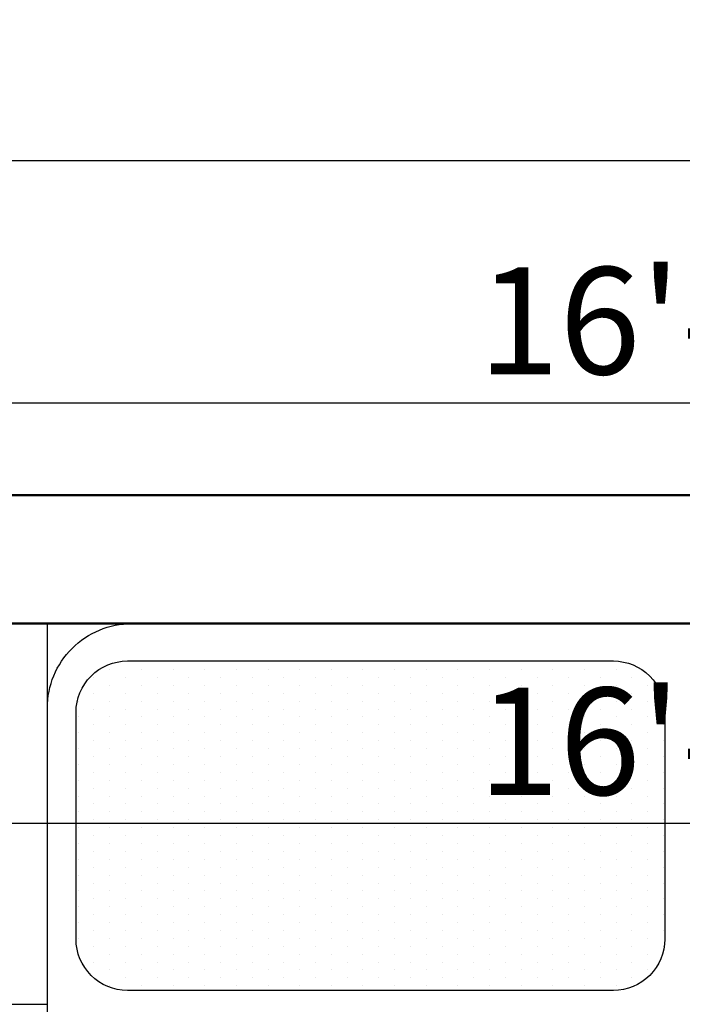
# Model space of a CAD drawing. Units: inches. Extents: x 3064 to 19385, y 846 to 15425.
# Tile 105 of 108: x 7734 to 7765, y 1373 to 1419. Entities that reach past the tile are written whole.
import ezdxf

# ---------------------------------------------------------------- set-up
doc = ezdxf.new("R2010")
doc.units = ezdxf.units.IN
for name, color, linetype, lineweight in [('A-ANNO-DIMS', 2, 'Continuous', 18), ('A-FLOR-FIXT', 9, 'Continuous', 18), ('A-WALL', 7, 'Continuous', 50)]:
    doc.layers.add(name, color=color, linetype=linetype, lineweight=lineweight)
doc.layers.add('BLOCK', color=6, linetype='Continuous')
doc.styles.get("Standard").update_dxf_attribs({"font": 'arial.ttf'})
doc.dimstyles.new('ISO-25', dxfattribs={"dimtxt": 9, "dimasz": 2.5, "dimexe": 1.25, "dimexo": 0.625, "dimtad": 1, "dimdec": 1, "dimlunit": 3, "dimtxsty": 'Standard', "dimcen": 2.5, "dimadec": 0, "dimazin": 0, "dimtfac": 1, "dimtdec": 1, "dimtmove": 0, "dimatfit": 3, "dimfxl": 1, "dimarcsym": 0})

# ---------------------------------------------------------------- blocks, each defined once
blk = doc.blocks.new('*D338')
at = {"layer": 'A-ANNO-DIMS', "color": 0, "lineweight": -2, "transparency": 16777216}
for p, q in [((7667.246, 1396.965), (7667.246, 1401.902)), ((7862.246, 1396.965), (7862.246, 1401.902)), ((7669.746, 1400.652), (7859.746, 1400.652))]:
    blk.add_line(p, q, dxfattribs=at)
at = {"layer": 'A-ANNO-DIMS', "color": 0, "transparency": 16777216}
for points in [[(7669.746, 1401.069), (7669.746, 1400.235), (7667.246, 1400.652)], [(7859.746, 1401.069), (7859.746, 1400.235), (7862.246, 1400.652)]]:
    blk.add_solid(points, dxfattribs=at)
at = {"layer": 'Defpoints', "color": 0, "transparency": 16777216}
for p in [(7862.246, 1400.652), (7667.246, 1396.34), (7862.246, 1396.34)]:
    blk.add_point(p, dxfattribs=at)
at = {"layer": 'A-ANNO-DIMS', "color": 0, "transparency": 16777216, "insert": (7764.746, 1403.832), "char_height": 5, "attachment_point": 5}
blk.add_mtext('16\'-3"', dxfattribs=at)
blk = doc.blocks.new('*D226')
at = {"layer": 'A-ANNO-DIMS', "color": 0, "lineweight": -2, "transparency": 16777216}
for p, q in [((7526.246, 1396.965), (7526.246, 1413.199)), ((7868.246, 1396.965), (7868.246, 1413.199)), ((7865.746, 1411.949), (7528.746, 1411.949))]:
    blk.add_line(p, q, dxfattribs=at)
at = {"layer": 'A-ANNO-DIMS', "color": 0, "transparency": 16777216}
for points in [[(7528.746, 1412.366), (7528.746, 1411.533), (7526.246, 1411.949)], [(7865.746, 1412.366), (7865.746, 1411.533), (7868.246, 1411.949)]]:
    blk.add_solid(points, dxfattribs=at)
at = {"layer": 'Defpoints', "color": 0, "transparency": 16777216}
for p in [(7526.246, 1411.949), (7526.246, 1396.34), (7868.246, 1396.34)]:
    blk.add_point(p, dxfattribs=at)
at = {"layer": 'A-ANNO-DIMS', "color": 0, "transparency": 16777216, "insert": (7697.246, 1415.127), "char_height": 5, "attachment_point": 5}
blk.add_mtext('28\'-6"', dxfattribs=at)
blk = doc.blocks.new('*D248')
at = {"layer": 'A-ANNO-DIMS', "color": 0, "lineweight": -2, "transparency": 16777216}
for p, q in [((7667.246, 1389.715), (7667.246, 1379.771)), ((7862.246, 1389.715), (7862.246, 1379.771)), ((7669.746, 1381.021), (7859.746, 1381.021))]:
    blk.add_line(p, q, dxfattribs=at)
at = {"layer": 'A-ANNO-DIMS', "color": 0, "transparency": 16777216}
for points in [[(7669.746, 1381.437), (7669.746, 1380.604), (7667.246, 1381.021)], [(7859.746, 1381.437), (7859.746, 1380.604), (7862.246, 1381.021)]]:
    blk.add_solid(points, dxfattribs=at)
at = {"layer": 'Defpoints', "color": 0, "transparency": 16777216}
for p in [(7667.246, 1390.34), (7862.246, 1390.34), (7862.246, 1381.021)]:
    blk.add_point(p, dxfattribs=at)
at = {"layer": 'A-ANNO-DIMS', "color": 0, "transparency": 16777216, "insert": (7764.746, 1384.2), "char_height": 5, "attachment_point": 5}
blk.add_mtext('16\'-3"', dxfattribs=at)
blk = doc.blocks.new('*X7')
at = {"color": 0}
for p, q in [((266.4375, 457.03125), (266.4375, 457.03125)), ((266.8125, 457.03125), (266.8125, 457.03125)), ((267.1875, 457.03125), (267.1875, 457.03125)), ((267.5625, 457.03125), (267.5625, 457.03125)), ((267.9375, 457.03125), (267.9375, 457.03125)), ((268.3125, 457.03125), (268.3125, 457.03125)), ((268.6875, 457.03125), (268.6875, 457.03125)), ((269.0625, 457.03125), (269.0625, 457.03125)), ((269.4375, 457.03125), (269.4375, 457.03125)), ((269.8125, 457.03125), (269.8125, 457.03125)), ((270.1875, 457.03125), (270.1875, 457.03125)), ((270.5625, 457.03125), (270.5625, 457.03125)), ((270.9375, 457.03125), (270.9375, 457.03125)), ((271.3125, 457.03125), (271.3125, 457.03125)), ((271.6875, 457.03125), (271.6875, 457.03125)), ((272.0625, 457.03125), (272.0625, 457.03125)), ((266.25, 456.9375), (266.25, 456.9375)), ((266.625, 456.9375), (266.625, 456.9375)), ((267, 456.9375), (267, 456.9375)), ((267.375, 456.9375), (267.375, 456.9375)), ((267.75, 456.9375), (267.75, 456.9375)), ((268.125, 456.9375), (268.125, 456.9375)), ((268.5, 456.9375), (268.5, 456.9375)), ((268.875, 456.9375), (268.875, 456.9375)), ((269.25, 456.9375), (269.25, 456.9375)), ((269.625, 456.9375), (269.625, 456.9375)), ((270, 456.9375), (270, 456.9375)), ((270.375, 456.9375), (270.375, 456.9375)), ((270.75, 456.9375), (270.75, 456.9375)), ((271.125, 456.9375), (271.125, 456.9375)), ((271.5, 456.9375), (271.5, 456.9375)), ((271.875, 456.9375), (271.875, 456.9375)), ((272.25, 456.9375), (272.25, 456.9375)), ((266.0625, 456.84375), (266.0625, 456.84375)), ((266.25, 456.75), (266.25, 456.75)), ((266.4375, 456.84375), (266.4375, 456.84375)), ((266.625, 456.75), (266.625, 456.75)), ((266.8125, 456.84375), (266.8125, 456.84375)), ((267, 456.75), (267, 456.75)), ((267.1875, 456.84375), (267.1875, 456.84375)), ((267.375, 456.75), (267.375, 456.75)), ((267.5625, 456.84375), (267.5625, 456.84375)), ((267.75, 456.75), (267.75, 456.75)), ((267.9375, 456.84375), (267.9375, 456.84375)), ((268.125, 456.75), (268.125, 456.75)), ((268.3125, 456.84375), (268.3125, 456.84375)), ((268.5, 456.75), (268.5, 456.75)), ((268.6875, 456.84375), (268.6875, 456.84375)), ((268.875, 456.75), (268.875, 456.75)), ((269.0625, 456.84375), (269.0625, 456.84375)), ((269.25, 456.75), (269.25, 456.75)), ((269.4375, 456.84375), (269.4375, 456.84375)), ((269.625, 456.75), (269.625, 456.75)), ((269.8125, 456.84375), (269.8125, 456.84375)), ((270, 456.75), (270, 456.75)), ((270.1875, 456.84375), (270.1875, 456.84375)), ((270.375, 456.75), (270.375, 456.75)), ((270.5625, 456.84375), (270.5625, 456.84375)), ((270.75, 456.75), (270.75, 456.75)), ((270.9375, 456.84375), (270.9375, 456.84375)), ((271.125, 456.75), (271.125, 456.75)), ((271.3125, 456.84375), (271.3125, 456.84375)), ((271.5, 456.75), (271.5, 456.75)), ((271.6875, 456.84375), (271.6875, 456.84375)), ((271.875, 456.75), (271.875, 456.75)), ((272.0625, 456.84375), (272.0625, 456.84375)), ((272.25, 456.75), (272.25, 456.75)), ((272.4375, 456.84375), (272.4375, 456.84375)), ((272.625, 456.75), (272.625, 456.75)), ((266.0625, 456.65625), (266.0625, 456.65625)), ((266.4375, 456.65625), (266.4375, 456.65625)), ((266.8125, 456.65625), (266.8125, 456.65625)), ((267.1875, 456.65625), (267.1875, 456.65625)), ((267.5625, 456.65625), (267.5625, 456.65625)), ((267.9375, 456.65625), (267.9375, 456.65625)), ((268.3125, 456.65625), (268.3125, 456.65625)), ((268.6875, 456.65625), (268.6875, 456.65625)), ((269.0625, 456.65625), (269.0625, 456.65625)), ((269.4375, 456.65625), (269.4375, 456.65625)), ((269.8125, 456.65625), (269.8125, 456.65625)), ((270.1875, 456.65625), (270.1875, 456.65625)), ((270.5625, 456.65625), (270.5625, 456.65625)), ((270.9375, 456.65625), (270.9375, 456.65625)), ((271.3125, 456.65625), (271.3125, 456.65625)), ((271.6875, 456.65625), (271.6875, 456.65625)), ((272.0625, 456.65625), (272.0625, 456.65625)), ((272.4375, 456.65625), (272.4375, 456.65625)), ((265.875, 456.5625), (265.875, 456.5625)), ((266.25, 456.5625), (266.25, 456.5625)), ((266.625, 456.5625), (266.625, 456.5625)), ((267, 456.5625), (267, 456.5625)), ((267.375, 456.5625), (267.375, 456.5625)), ((267.75, 456.5625), (267.75, 456.5625)), ((268.125, 456.5625), (268.125, 456.5625)), ((268.5, 456.5625), (268.5, 456.5625)), ((268.875, 456.5625), (268.875, 456.5625)), ((269.25, 456.5625), (269.25, 456.5625)), ((269.625, 456.5625), (269.625, 456.5625)), ((270, 456.5625), (270, 456.5625)), ((270.375, 456.5625), (270.375, 456.5625)), ((270.75, 456.5625), (270.75, 456.5625)), ((271.125, 456.5625), (271.125, 456.5625)), ((271.5, 456.5625), (271.5, 456.5625)), ((271.875, 456.5625), (271.875, 456.5625)), ((272.25, 456.5625), (272.25, 456.5625)), ((272.625, 456.5625), (272.625, 456.5625)), ((266.0625, 456.46875), (266.0625, 456.46875)), ((266.4375, 456.46875), (266.4375, 456.46875)), ((266.8125, 456.46875), (266.8125, 456.46875)), ((267.1875, 456.46875), (267.1875, 456.46875)), ((267.5625, 456.46875), (267.5625, 456.46875)), ((267.9375, 456.46875), (267.9375, 456.46875)), ((268.3125, 456.46875), (268.3125, 456.46875)), ((268.6875, 456.46875), (268.6875, 456.46875)), ((269.0625, 456.46875), (269.0625, 456.46875)), ((269.4375, 456.46875), (269.4375, 456.46875)), ((269.8125, 456.46875), (269.8125, 456.46875)), ((270.1875, 456.46875), (270.1875, 456.46875)), ((270.5625, 456.46875), (270.5625, 456.46875)), ((270.9375, 456.46875), (270.9375, 456.46875)), ((271.3125, 456.46875), (271.3125, 456.46875)), ((271.6875, 456.46875), (271.6875, 456.46875)), ((272.0625, 456.46875), (272.0625, 456.46875)), ((272.4375, 456.46875), (272.4375, 456.46875)), ((272.8125, 456.46875), (272.8125, 456.46875)), ((265.875, 456.375), (265.875, 456.375)), ((266.0625, 456.28125), (266.0625, 456.28125)), ((266.25, 456.375), (266.25, 456.375)), ((266.4375, 456.28125), (266.4375, 456.28125)), ((266.625, 456.375), (266.625, 456.375)), ((266.8125, 456.28125), (266.8125, 456.28125)), ((267, 456.375), (267, 456.375)), ((267.1875, 456.28125), (267.1875, 456.28125)), ((267.375, 456.375), (267.375, 456.375)), ((267.5625, 456.28125), (267.5625, 456.28125)), ((267.75, 456.375), (267.75, 456.375)), ((267.9375, 456.28125), (267.9375, 456.28125)), ((268.125, 456.375), (268.125, 456.375)), ((268.3125, 456.28125), (268.3125, 456.28125)), ((268.5, 456.375), (268.5, 456.375)), ((268.6875, 456.28125), (268.6875, 456.28125)), ((268.875, 456.375), (268.875, 456.375)), ((269.0625, 456.28125), (269.0625, 456.28125)), ((269.25, 456.375), (269.25, 456.375)), ((269.4375, 456.28125), (269.4375, 456.28125)), ((269.625, 456.375), (269.625, 456.375)), ((269.8125, 456.28125), (269.8125, 456.28125)), ((270, 456.375), (270, 456.375)), ((270.1875, 456.28125), (270.1875, 456.28125)), ((270.375, 456.375), (270.375, 456.375)), ((270.5625, 456.28125), (270.5625, 456.28125)), ((270.75, 456.375), (270.75, 456.375)), ((270.9375, 456.28125), (270.9375, 456.28125)), ((271.125, 456.375), (271.125, 456.375)), ((271.3125, 456.28125), (271.3125, 456.28125)), ((271.5, 456.375), (271.5, 456.375)), ((271.6875, 456.28125), (271.6875, 456.28125)), ((271.875, 456.375), (271.875, 456.375)), ((272.0625, 456.28125), (272.0625, 456.28125)), ((272.25, 456.375), (272.25, 456.375)), ((272.4375, 456.28125), (272.4375, 456.28125)), ((272.625, 456.375), (272.625, 456.375)), ((272.8125, 456.28125), (272.8125, 456.28125)), ((265.875, 456.1875), (265.875, 456.1875)), ((266.25, 456.1875), (266.25, 456.1875)), ((266.625, 456.1875), (266.625, 456.1875)), ((267, 456.1875), (267, 456.1875)), ((267.375, 456.1875), (267.375, 456.1875)), ((267.75, 456.1875), (267.75, 456.1875)), ((268.125, 456.1875), (268.125, 456.1875)), ((268.5, 456.1875), (268.5, 456.1875)), ((268.875, 456.1875), (268.875, 456.1875)), ((269.25, 456.1875), (269.25, 456.1875)), ((269.625, 456.1875), (269.625, 456.1875)), ((270, 456.1875), (270, 456.1875)), ((270.375, 456.1875), (270.375, 456.1875)), ((270.75, 456.1875), (270.75, 456.1875)), ((271.125, 456.1875), (271.125, 456.1875)), ((271.5, 456.1875), (271.5, 456.1875)), ((271.875, 456.1875), (271.875, 456.1875)), ((272.25, 456.1875), (272.25, 456.1875)), ((272.625, 456.1875), (272.625, 456.1875)), ((266.0625, 456.09375), (266.0625, 456.09375)), ((266.4375, 456.09375), (266.4375, 456.09375)), ((266.8125, 456.09375), (266.8125, 456.09375)), ((267.1875, 456.09375), (267.1875, 456.09375)), ((267.5625, 456.09375), (267.5625, 456.09375)), ((267.9375, 456.09375), (267.9375, 456.09375)), ((268.3125, 456.09375), (268.3125, 456.09375)), ((268.6875, 456.09375), (268.6875, 456.09375)), ((269.0625, 456.09375), (269.0625, 456.09375)), ((269.4375, 456.09375), (269.4375, 456.09375)), ((269.8125, 456.09375), (269.8125, 456.09375)), ((270.1875, 456.09375), (270.1875, 456.09375)), ((270.5625, 456.09375), (270.5625, 456.09375)), ((270.9375, 456.09375), (270.9375, 456.09375)), ((271.3125, 456.09375), (271.3125, 456.09375)), ((271.6875, 456.09375), (271.6875, 456.09375)), ((272.0625, 456.09375), (272.0625, 456.09375)), ((272.4375, 456.09375), (272.4375, 456.09375)), ((272.8125, 456.09375), (272.8125, 456.09375)), ((265.875, 456), (265.875, 456)), ((266.25, 456), (266.25, 456)), ((266.625, 456), (266.625, 456)), ((267, 456), (267, 456)), ((267.375, 456), (267.375, 456)), ((267.75, 456), (267.75, 456)), ((268.125, 456), (268.125, 456)), ((268.5, 456), (268.5, 456)), ((268.875, 456), (268.875, 456)), ((269.25, 456), (269.25, 456)), ((269.625, 456), (269.625, 456)), ((270, 456), (270, 456)), ((270.375, 456), (270.375, 456)), ((270.75, 456), (270.75, 456)), ((271.125, 456), (271.125, 456)), ((271.5, 456), (271.5, 456)), ((271.875, 456), (271.875, 456)), ((272.25, 456), (272.25, 456)), ((272.625, 456), (272.625, 456)), ((265.875, 455.8125), (265.875, 455.8125)), ((266.0625, 455.90625), (266.0625, 455.90625)), ((266.25, 455.8125), (266.25, 455.8125)), ((266.4375, 455.90625), (266.4375, 455.90625)), ((266.625, 455.8125), (266.625, 455.8125)), ((266.8125, 455.90625), (266.8125, 455.90625)), ((267, 455.8125), (267, 455.8125)), ((267.1875, 455.90625), (267.1875, 455.90625)), ((267.375, 455.8125), (267.375, 455.8125)), ((267.5625, 455.90625), (267.5625, 455.90625)), ((267.75, 455.8125), (267.75, 455.8125)), ((267.9375, 455.90625), (267.9375, 455.90625)), ((268.125, 455.8125), (268.125, 455.8125)), ((268.3125, 455.90625), (268.3125, 455.90625)), ((268.5, 455.8125), (268.5, 455.8125)), ((268.6875, 455.90625), (268.6875, 455.90625)), ((268.875, 455.8125), (268.875, 455.8125)), ((269.0625, 455.90625), (269.0625, 455.90625)), ((269.25, 455.8125), (269.25, 455.8125)), ((269.4375, 455.90625), (269.4375, 455.90625)), ((269.625, 455.8125), (269.625, 455.8125)), ((269.8125, 455.90625), (269.8125, 455.90625)), ((270, 455.8125), (270, 455.8125)), ((270.1875, 455.90625), (270.1875, 455.90625)), ((270.375, 455.8125), (270.375, 455.8125)), ((270.5625, 455.90625), (270.5625, 455.90625)), ((270.75, 455.8125), (270.75, 455.8125)), ((270.9375, 455.90625), (270.9375, 455.90625)), ((271.125, 455.8125), (271.125, 455.8125)), ((271.3125, 455.90625), (271.3125, 455.90625)), ((271.5, 455.8125), (271.5, 455.8125)), ((271.6875, 455.90625), (271.6875, 455.90625)), ((271.875, 455.8125), (271.875, 455.8125)), ((272.0625, 455.90625), (272.0625, 455.90625)), ((272.25, 455.8125), (272.25, 455.8125)), ((272.4375, 455.90625), (272.4375, 455.90625)), ((272.625, 455.8125), (272.625, 455.8125)), ((272.8125, 455.90625), (272.8125, 455.90625)), ((266.0625, 455.71875), (266.0625, 455.71875)), ((266.4375, 455.71875), (266.4375, 455.71875)), ((266.8125, 455.71875), (266.8125, 455.71875)), ((267.1875, 455.71875), (267.1875, 455.71875)), ((267.5625, 455.71875), (267.5625, 455.71875)), ((267.9375, 455.71875), (267.9375, 455.71875)), ((268.3125, 455.71875), (268.3125, 455.71875)), ((268.6875, 455.71875), (268.6875, 455.71875)), ((269.0625, 455.71875), (269.0625, 455.71875)), ((269.4375, 455.71875), (269.4375, 455.71875)), ((269.8125, 455.71875), (269.8125, 455.71875)), ((270.1875, 455.71875), (270.1875, 455.71875)), ((270.5625, 455.71875), (270.5625, 455.71875)), ((270.9375, 455.71875), (270.9375, 455.71875)), ((271.3125, 455.71875), (271.3125, 455.71875)), ((271.6875, 455.71875), (271.6875, 455.71875)), ((272.0625, 455.71875), (272.0625, 455.71875)), ((272.4375, 455.71875), (272.4375, 455.71875)), ((272.8125, 455.71875), (272.8125, 455.71875)), ((265.875, 455.625), (265.875, 455.625)), ((266.25, 455.625), (266.25, 455.625)), ((266.625, 455.625), (266.625, 455.625)), ((267, 455.625), (267, 455.625)), ((267.375, 455.625), (267.375, 455.625)), ((267.75, 455.625), (267.75, 455.625)), ((268.125, 455.625), (268.125, 455.625)), ((268.5, 455.625), (268.5, 455.625)), ((268.875, 455.625), (268.875, 455.625)), ((269.25, 455.625), (269.25, 455.625)), ((269.625, 455.625), (269.625, 455.625)), ((270, 455.625), (270, 455.625)), ((270.375, 455.625), (270.375, 455.625)), ((270.75, 455.625), (270.75, 455.625)), ((271.125, 455.625), (271.125, 455.625)), ((271.5, 455.625), (271.5, 455.625)), ((271.875, 455.625), (271.875, 455.625)), ((272.25, 455.625), (272.25, 455.625)), ((272.625, 455.625), (272.625, 455.625)), ((266.0625, 455.53125), (266.0625, 455.53125)), ((266.4375, 455.53125), (266.4375, 455.53125)), ((266.8125, 455.53125), (266.8125, 455.53125)), ((267.1875, 455.53125), (267.1875, 455.53125)), ((267.5625, 455.53125), (267.5625, 455.53125)), ((267.9375, 455.53125), (267.9375, 455.53125)), ((268.3125, 455.53125), (268.3125, 455.53125)), ((268.6875, 455.53125), (268.6875, 455.53125)), ((269.0625, 455.53125), (269.0625, 455.53125)), ((269.4375, 455.53125), (269.4375, 455.53125)), ((269.8125, 455.53125), (269.8125, 455.53125)), ((270.1875, 455.53125), (270.1875, 455.53125)), ((270.5625, 455.53125), (270.5625, 455.53125)), ((270.9375, 455.53125), (270.9375, 455.53125)), ((271.3125, 455.53125), (271.3125, 455.53125)), ((271.6875, 455.53125), (271.6875, 455.53125)), ((272.0625, 455.53125), (272.0625, 455.53125)), ((272.4375, 455.53125), (272.4375, 455.53125)), ((272.8125, 455.53125), (272.8125, 455.53125)), ((265.875, 455.4375), (265.875, 455.4375)), ((266.0625, 455.34375), (266.0625, 455.34375)), ((266.25, 455.4375), (266.25, 455.4375)), ((266.4375, 455.34375), (266.4375, 455.34375)), ((266.625, 455.4375), (266.625, 455.4375)), ((266.8125, 455.34375), (266.8125, 455.34375)), ((267, 455.4375), (267, 455.4375)), ((267.1875, 455.34375), (267.1875, 455.34375)), ((267.375, 455.4375), (267.375, 455.4375)), ((267.5625, 455.34375), (267.5625, 455.34375)), ((267.75, 455.4375), (267.75, 455.4375)), ((267.9375, 455.34375), (267.9375, 455.34375)), ((268.125, 455.4375), (268.125, 455.4375)), ((268.3125, 455.34375), (268.3125, 455.34375)), ((268.5, 455.4375), (268.5, 455.4375)), ((268.6875, 455.34375), (268.6875, 455.34375)), ((268.875, 455.4375), (268.875, 455.4375)), ((269.0625, 455.34375), (269.0625, 455.34375)), ((269.25, 455.4375), (269.25, 455.4375)), ((269.4375, 455.34375), (269.4375, 455.34375)), ((269.625, 455.4375), (269.625, 455.4375)), ((269.8125, 455.34375), (269.8125, 455.34375)), ((270, 455.4375), (270, 455.4375)), ((270.1875, 455.34375), (270.1875, 455.34375)), ((270.375, 455.4375), (270.375, 455.4375)), ((270.5625, 455.34375), (270.5625, 455.34375)), ((270.75, 455.4375), (270.75, 455.4375)), ((270.9375, 455.34375), (270.9375, 455.34375)), ((271.125, 455.4375), (271.125, 455.4375)), ((271.3125, 455.34375), (271.3125, 455.34375)), ((271.5, 455.4375), (271.5, 455.4375)), ((271.6875, 455.34375), (271.6875, 455.34375)), ((271.875, 455.4375), (271.875, 455.4375)), ((272.0625, 455.34375), (272.0625, 455.34375)), ((272.25, 455.4375), (272.25, 455.4375)), ((272.4375, 455.34375), (272.4375, 455.34375)), ((272.625, 455.4375), (272.625, 455.4375)), ((272.8125, 455.34375), (272.8125, 455.34375)), ((265.875, 455.25), (265.875, 455.25)), ((266.25, 455.25), (266.25, 455.25)), ((266.625, 455.25), (266.625, 455.25)), ((267, 455.25), (267, 455.25)), ((267.375, 455.25), (267.375, 455.25)), ((267.75, 455.25), (267.75, 455.25)), ((268.125, 455.25), (268.125, 455.25)), ((268.5, 455.25), (268.5, 455.25)), ((268.875, 455.25), (268.875, 455.25)), ((269.25, 455.25), (269.25, 455.25)), ((269.625, 455.25), (269.625, 455.25)), ((270, 455.25), (270, 455.25)), ((270.375, 455.25), (270.375, 455.25)), ((270.75, 455.25), (270.75, 455.25)), ((271.125, 455.25), (271.125, 455.25)), ((271.5, 455.25), (271.5, 455.25)), ((271.875, 455.25), (271.875, 455.25)), ((272.25, 455.25), (272.25, 455.25)), ((272.625, 455.25), (272.625, 455.25)), ((266.0625, 455.15625), (266.0625, 455.15625)), ((266.4375, 455.15625), (266.4375, 455.15625)), ((266.8125, 455.15625), (266.8125, 455.15625)), ((267.1875, 455.15625), (267.1875, 455.15625)), ((267.5625, 455.15625), (267.5625, 455.15625)), ((267.9375, 455.15625), (267.9375, 455.15625)), ((268.3125, 455.15625), (268.3125, 455.15625)), ((268.6875, 455.15625), (268.6875, 455.15625)), ((269.0625, 455.15625), (269.0625, 455.15625)), ((269.4375, 455.15625), (269.4375, 455.15625)), ((269.8125, 455.15625), (269.8125, 455.15625)), ((270.1875, 455.15625), (270.1875, 455.15625)), ((270.5625, 455.15625), (270.5625, 455.15625)), ((270.9375, 455.15625), (270.9375, 455.15625)), ((271.3125, 455.15625), (271.3125, 455.15625)), ((271.6875, 455.15625), (271.6875, 455.15625)), ((272.0625, 455.15625), (272.0625, 455.15625)), ((272.4375, 455.15625), (272.4375, 455.15625)), ((272.8125, 455.15625), (272.8125, 455.15625)), ((265.875, 455.0625), (265.875, 455.0625)), ((266.25, 455.0625), (266.25, 455.0625)), ((266.625, 455.0625), (266.625, 455.0625)), ((267, 455.0625), (267, 455.0625)), ((267.375, 455.0625), (267.375, 455.0625)), ((267.75, 455.0625), (267.75, 455.0625)), ((268.125, 455.0625), (268.125, 455.0625)), ((268.5, 455.0625), (268.5, 455.0625)), ((268.875, 455.0625), (268.875, 455.0625)), ((269.25, 455.0625), (269.25, 455.0625)), ((269.625, 455.0625), (269.625, 455.0625)), ((270, 455.0625), (270, 455.0625)), ((270.375, 455.0625), (270.375, 455.0625)), ((270.75, 455.0625), (270.75, 455.0625)), ((271.125, 455.0625), (271.125, 455.0625)), ((271.5, 455.0625), (271.5, 455.0625)), ((271.875, 455.0625), (271.875, 455.0625)), ((272.25, 455.0625), (272.25, 455.0625)), ((272.625, 455.0625), (272.625, 455.0625)), ((265.875, 454.875), (265.875, 454.875)), ((266.0625, 454.96875), (266.0625, 454.96875)), ((266.25, 454.875), (266.25, 454.875)), ((266.4375, 454.96875), (266.4375, 454.96875)), ((266.625, 454.875), (266.625, 454.875)), ((266.8125, 454.96875), (266.8125, 454.96875)), ((267, 454.875), (267, 454.875)), ((267.1875, 454.96875), (267.1875, 454.96875)), ((267.375, 454.875), (267.375, 454.875)), ((267.5625, 454.96875), (267.5625, 454.96875)), ((267.75, 454.875), (267.75, 454.875)), ((267.9375, 454.96875), (267.9375, 454.96875)), ((268.125, 454.875), (268.125, 454.875)), ((268.3125, 454.96875), (268.3125, 454.96875)), ((268.5, 454.875), (268.5, 454.875)), ((268.6875, 454.96875), (268.6875, 454.96875)), ((268.875, 454.875), (268.875, 454.875)), ((269.0625, 454.96875), (269.0625, 454.96875)), ((269.25, 454.875), (269.25, 454.875)), ((269.4375, 454.96875), (269.4375, 454.96875)), ((269.625, 454.875), (269.625, 454.875)), ((269.8125, 454.96875), (269.8125, 454.96875)), ((270, 454.875), (270, 454.875)), ((270.1875, 454.96875), (270.1875, 454.96875)), ((270.375, 454.875), (270.375, 454.875)), ((270.5625, 454.96875), (270.5625, 454.96875)), ((270.75, 454.875), (270.75, 454.875)), ((270.9375, 454.96875), (270.9375, 454.96875)), ((271.125, 454.875), (271.125, 454.875)), ((271.3125, 454.96875), (271.3125, 454.96875)), ((271.5, 454.875), (271.5, 454.875)), ((271.6875, 454.96875), (271.6875, 454.96875)), ((271.875, 454.875), (271.875, 454.875)), ((272.0625, 454.96875), (272.0625, 454.96875)), ((272.25, 454.875), (272.25, 454.875)), ((272.4375, 454.96875), (272.4375, 454.96875)), ((272.625, 454.875), (272.625, 454.875)), ((272.8125, 454.96875), (272.8125, 454.96875)), ((266.0625, 454.78125), (266.0625, 454.78125)), ((266.4375, 454.78125), (266.4375, 454.78125)), ((266.8125, 454.78125), (266.8125, 454.78125)), ((267.1875, 454.78125), (267.1875, 454.78125)), ((267.5625, 454.78125), (267.5625, 454.78125)), ((267.9375, 454.78125), (267.9375, 454.78125)), ((268.3125, 454.78125), (268.3125, 454.78125)), ((268.6875, 454.78125), (268.6875, 454.78125)), ((269.0625, 454.78125), (269.0625, 454.78125)), ((269.4375, 454.78125), (269.4375, 454.78125)), ((269.8125, 454.78125), (269.8125, 454.78125)), ((270.1875, 454.78125), (270.1875, 454.78125)), ((270.5625, 454.78125), (270.5625, 454.78125)), ((270.9375, 454.78125), (270.9375, 454.78125)), ((271.3125, 454.78125), (271.3125, 454.78125)), ((271.6875, 454.78125), (271.6875, 454.78125)), ((272.0625, 454.78125), (272.0625, 454.78125)), ((272.4375, 454.78125), (272.4375, 454.78125)), ((272.8125, 454.78125), (272.8125, 454.78125)), ((265.875, 454.6875), (265.875, 454.6875)), ((266.25, 454.6875), (266.25, 454.6875)), ((266.625, 454.6875), (266.625, 454.6875)), ((267, 454.6875), (267, 454.6875)), ((267.375, 454.6875), (267.375, 454.6875)), ((267.75, 454.6875), (267.75, 454.6875)), ((268.125, 454.6875), (268.125, 454.6875)), ((268.5, 454.6875), (268.5, 454.6875)), ((268.875, 454.6875), (268.875, 454.6875)), ((269.25, 454.6875), (269.25, 454.6875)), ((269.625, 454.6875), (269.625, 454.6875)), ((270, 454.6875), (270, 454.6875)), ((270.375, 454.6875), (270.375, 454.6875)), ((270.75, 454.6875), (270.75, 454.6875)), ((271.125, 454.6875), (271.125, 454.6875)), ((271.5, 454.6875), (271.5, 454.6875)), ((271.875, 454.6875), (271.875, 454.6875)), ((272.25, 454.6875), (272.25, 454.6875)), ((272.625, 454.6875), (272.625, 454.6875)), ((266.0625, 454.59375), (266.0625, 454.59375)), ((266.4375, 454.59375), (266.4375, 454.59375)), ((266.8125, 454.59375), (266.8125, 454.59375)), ((267.1875, 454.59375), (267.1875, 454.59375)), ((267.5625, 454.59375), (267.5625, 454.59375)), ((267.9375, 454.59375), (267.9375, 454.59375)), ((268.3125, 454.59375), (268.3125, 454.59375)), ((268.6875, 454.59375), (268.6875, 454.59375)), ((269.0625, 454.59375), (269.0625, 454.59375)), ((269.4375, 454.59375), (269.4375, 454.59375)), ((269.8125, 454.59375), (269.8125, 454.59375)), ((270.1875, 454.59375), (270.1875, 454.59375)), ((270.5625, 454.59375), (270.5625, 454.59375)), ((270.9375, 454.59375), (270.9375, 454.59375)), ((271.3125, 454.59375), (271.3125, 454.59375)), ((271.6875, 454.59375), (271.6875, 454.59375)), ((272.0625, 454.59375), (272.0625, 454.59375)), ((272.4375, 454.59375), (272.4375, 454.59375)), ((272.8125, 454.59375), (272.8125, 454.59375)), ((265.875, 454.5), (265.875, 454.5)), ((266.0625, 454.40625), (266.0625, 454.40625)), ((266.25, 454.5), (266.25, 454.5)), ((266.4375, 454.40625), (266.4375, 454.40625)), ((266.625, 454.5), (266.625, 454.5)), ((266.8125, 454.40625), (266.8125, 454.40625)), ((267, 454.5), (267, 454.5)), ((267.1875, 454.40625), (267.1875, 454.40625)), ((267.375, 454.5), (267.375, 454.5)), ((267.5625, 454.40625), (267.5625, 454.40625)), ((267.75, 454.5), (267.75, 454.5)), ((267.9375, 454.40625), (267.9375, 454.40625)), ((268.125, 454.5), (268.125, 454.5)), ((268.3125, 454.40625), (268.3125, 454.40625)), ((268.5, 454.5), (268.5, 454.5)), ((268.6875, 454.40625), (268.6875, 454.40625)), ((268.875, 454.5), (268.875, 454.5)), ((269.0625, 454.40625), (269.0625, 454.40625)), ((269.25, 454.5), (269.25, 454.5)), ((269.4375, 454.40625), (269.4375, 454.40625)), ((269.625, 454.5), (269.625, 454.5)), ((269.8125, 454.40625), (269.8125, 454.40625)), ((270, 454.5), (270, 454.5)), ((270.1875, 454.40625), (270.1875, 454.40625)), ((270.375, 454.5), (270.375, 454.5)), ((270.5625, 454.40625), (270.5625, 454.40625)), ((270.75, 454.5), (270.75, 454.5)), ((270.9375, 454.40625), (270.9375, 454.40625)), ((271.125, 454.5), (271.125, 454.5)), ((271.3125, 454.40625), (271.3125, 454.40625)), ((271.5, 454.5), (271.5, 454.5)), ((271.6875, 454.40625), (271.6875, 454.40625)), ((271.875, 454.5), (271.875, 454.5)), ((272.0625, 454.40625), (272.0625, 454.40625)), ((272.25, 454.5), (272.25, 454.5)), ((272.4375, 454.40625), (272.4375, 454.40625)), ((272.625, 454.5), (272.625, 454.5)), ((272.8125, 454.40625), (272.8125, 454.40625)), ((265.875, 454.3125), (265.875, 454.3125)), ((266.25, 454.3125), (266.25, 454.3125)), ((266.625, 454.3125), (266.625, 454.3125)), ((267, 454.3125), (267, 454.3125)), ((267.375, 454.3125), (267.375, 454.3125)), ((267.75, 454.3125), (267.75, 454.3125)), ((268.125, 454.3125), (268.125, 454.3125)), ((268.5, 454.3125), (268.5, 454.3125)), ((268.875, 454.3125), (268.875, 454.3125)), ((269.25, 454.3125), (269.25, 454.3125)), ((269.625, 454.3125), (269.625, 454.3125)), ((270, 454.3125), (270, 454.3125)), ((270.375, 454.3125), (270.375, 454.3125)), ((270.75, 454.3125), (270.75, 454.3125)), ((271.125, 454.3125), (271.125, 454.3125)), ((271.5, 454.3125), (271.5, 454.3125)), ((271.875, 454.3125), (271.875, 454.3125)), ((272.25, 454.3125), (272.25, 454.3125)), ((272.625, 454.3125), (272.625, 454.3125)), ((266.0625, 454.21875), (266.0625, 454.21875)), ((266.4375, 454.21875), (266.4375, 454.21875)), ((266.8125, 454.21875), (266.8125, 454.21875)), ((267.1875, 454.21875), (267.1875, 454.21875)), ((267.5625, 454.21875), (267.5625, 454.21875)), ((267.9375, 454.21875), (267.9375, 454.21875)), ((268.3125, 454.21875), (268.3125, 454.21875)), ((268.6875, 454.21875), (268.6875, 454.21875)), ((269.0625, 454.21875), (269.0625, 454.21875)), ((269.4375, 454.21875), (269.4375, 454.21875)), ((269.8125, 454.21875), (269.8125, 454.21875)), ((270.1875, 454.21875), (270.1875, 454.21875)), ((270.5625, 454.21875), (270.5625, 454.21875)), ((270.9375, 454.21875), (270.9375, 454.21875)), ((271.3125, 454.21875), (271.3125, 454.21875)), ((271.6875, 454.21875), (271.6875, 454.21875)), ((272.0625, 454.21875), (272.0625, 454.21875)), ((272.4375, 454.21875), (272.4375, 454.21875)), ((272.8125, 454.21875), (272.8125, 454.21875)), ((265.875, 454.125), (265.875, 454.125)), ((266.25, 454.125), (266.25, 454.125)), ((266.625, 454.125), (266.625, 454.125)), ((267, 454.125), (267, 454.125)), ((267.375, 454.125), (267.375, 454.125)), ((267.75, 454.125), (267.75, 454.125)), ((268.125, 454.125), (268.125, 454.125)), ((268.5, 454.125), (268.5, 454.125)), ((268.875, 454.125), (268.875, 454.125)), ((269.25, 454.125), (269.25, 454.125)), ((269.625, 454.125), (269.625, 454.125)), ((270, 454.125), (270, 454.125)), ((270.375, 454.125), (270.375, 454.125)), ((270.75, 454.125), (270.75, 454.125)), ((271.125, 454.125), (271.125, 454.125)), ((271.5, 454.125), (271.5, 454.125)), ((271.875, 454.125), (271.875, 454.125)), ((272.25, 454.125), (272.25, 454.125)), ((272.625, 454.125), (272.625, 454.125)), ((265.875, 453.9375), (265.875, 453.9375)), ((266.0625, 454.03125), (266.0625, 454.03125)), ((266.25, 453.9375), (266.25, 453.9375)), ((266.4375, 454.03125), (266.4375, 454.03125)), ((266.625, 453.9375), (266.625, 453.9375)), ((266.8125, 454.03125), (266.8125, 454.03125)), ((267, 453.9375), (267, 453.9375)), ((267.1875, 454.03125), (267.1875, 454.03125)), ((267.375, 453.9375), (267.375, 453.9375)), ((267.5625, 454.03125), (267.5625, 454.03125)), ((267.75, 453.9375), (267.75, 453.9375)), ((267.9375, 454.03125), (267.9375, 454.03125)), ((268.125, 453.9375), (268.125, 453.9375)), ((268.3125, 454.03125), (268.3125, 454.03125)), ((268.5, 453.9375), (268.5, 453.9375)), ((268.6875, 454.03125), (268.6875, 454.03125)), ((268.875, 453.9375), (268.875, 453.9375)), ((269.0625, 454.03125), (269.0625, 454.03125)), ((269.25, 453.9375), (269.25, 453.9375)), ((269.4375, 454.03125), (269.4375, 454.03125)), ((269.625, 453.9375), (269.625, 453.9375)), ((269.8125, 454.03125), (269.8125, 454.03125)), ((270, 453.9375), (270, 453.9375)), ((270.1875, 454.03125), (270.1875, 454.03125)), ((270.375, 453.9375), (270.375, 453.9375)), ((270.5625, 454.03125), (270.5625, 454.03125)), ((270.75, 453.9375), (270.75, 453.9375)), ((270.9375, 454.03125), (270.9375, 454.03125)), ((271.125, 453.9375), (271.125, 453.9375)), ((271.3125, 454.03125), (271.3125, 454.03125)), ((271.5, 453.9375), (271.5, 453.9375)), ((271.6875, 454.03125), (271.6875, 454.03125)), ((271.875, 453.9375), (271.875, 453.9375)), ((272.0625, 454.03125), (272.0625, 454.03125)), ((272.25, 453.9375), (272.25, 453.9375)), ((272.4375, 454.03125), (272.4375, 454.03125)), ((272.625, 453.9375), (272.625, 453.9375)), ((272.8125, 454.03125), (272.8125, 454.03125)), ((266.0625, 453.84375), (266.0625, 453.84375)), ((266.4375, 453.84375), (266.4375, 453.84375)), ((266.8125, 453.84375), (266.8125, 453.84375)), ((267.1875, 453.84375), (267.1875, 453.84375)), ((267.5625, 453.84375), (267.5625, 453.84375)), ((267.9375, 453.84375), (267.9375, 453.84375)), ((268.3125, 453.84375), (268.3125, 453.84375)), ((268.6875, 453.84375), (268.6875, 453.84375)), ((269.0625, 453.84375), (269.0625, 453.84375)), ((269.4375, 453.84375), (269.4375, 453.84375)), ((269.8125, 453.84375), (269.8125, 453.84375)), ((270.1875, 453.84375), (270.1875, 453.84375)), ((270.5625, 453.84375), (270.5625, 453.84375)), ((270.9375, 453.84375), (270.9375, 453.84375)), ((271.3125, 453.84375), (271.3125, 453.84375)), ((271.6875, 453.84375), (271.6875, 453.84375)), ((272.0625, 453.84375), (272.0625, 453.84375)), ((272.4375, 453.84375), (272.4375, 453.84375)), ((272.8125, 453.84375), (272.8125, 453.84375)), ((265.875, 453.75), (265.875, 453.75)), ((266.25, 453.75), (266.25, 453.75)), ((266.625, 453.75), (266.625, 453.75)), ((267, 453.75), (267, 453.75)), ((267.375, 453.75), (267.375, 453.75)), ((267.75, 453.75), (267.75, 453.75)), ((268.125, 453.75), (268.125, 453.75)), ((268.5, 453.75), (268.5, 453.75)), ((268.875, 453.75), (268.875, 453.75)), ((269.25, 453.75), (269.25, 453.75)), ((269.625, 453.75), (269.625, 453.75)), ((270, 453.75), (270, 453.75)), ((270.375, 453.75), (270.375, 453.75)), ((270.75, 453.75), (270.75, 453.75)), ((271.125, 453.75), (271.125, 453.75)), ((271.5, 453.75), (271.5, 453.75)), ((271.875, 453.75), (271.875, 453.75)), ((272.25, 453.75), (272.25, 453.75)), ((272.625, 453.75), (272.625, 453.75)), ((266.0625, 453.65625), (266.0625, 453.65625)), ((266.4375, 453.65625), (266.4375, 453.65625)), ((266.8125, 453.65625), (266.8125, 453.65625)), ((267.1875, 453.65625), (267.1875, 453.65625)), ((267.5625, 453.65625), (267.5625, 453.65625)), ((267.9375, 453.65625), (267.9375, 453.65625)), ((268.3125, 453.65625), (268.3125, 453.65625)), ((268.6875, 453.65625), (268.6875, 453.65625)), ((269.0625, 453.65625), (269.0625, 453.65625)), ((269.4375, 453.65625), (269.4375, 453.65625)), ((269.8125, 453.65625), (269.8125, 453.65625)), ((270.1875, 453.65625), (270.1875, 453.65625)), ((270.5625, 453.65625), (270.5625, 453.65625)), ((270.9375, 453.65625), (270.9375, 453.65625)), ((271.3125, 453.65625), (271.3125, 453.65625)), ((271.6875, 453.65625), (271.6875, 453.65625)), ((272.0625, 453.65625), (272.0625, 453.65625)), ((272.4375, 453.65625), (272.4375, 453.65625)), ((272.8125, 453.65625), (272.8125, 453.65625)), ((266.0625, 453.46875), (266.0625, 453.46875)), ((266.25, 453.5625), (266.25, 453.5625)), ((266.4375, 453.46875), (266.4375, 453.46875)), ((266.625, 453.5625), (266.625, 453.5625)), ((266.8125, 453.46875), (266.8125, 453.46875)), ((267, 453.5625), (267, 453.5625)), ((267.1875, 453.46875), (267.1875, 453.46875)), ((267.375, 453.5625), (267.375, 453.5625)), ((267.5625, 453.46875), (267.5625, 453.46875)), ((267.75, 453.5625), (267.75, 453.5625)), ((267.9375, 453.46875), (267.9375, 453.46875)), ((268.125, 453.5625), (268.125, 453.5625)), ((268.3125, 453.46875), (268.3125, 453.46875)), ((268.5, 453.5625), (268.5, 453.5625)), ((268.6875, 453.46875), (268.6875, 453.46875)), ((268.875, 453.5625), (268.875, 453.5625)), ((269.0625, 453.46875), (269.0625, 453.46875)), ((269.25, 453.5625), (269.25, 453.5625)), ((269.4375, 453.46875), (269.4375, 453.46875)), ((269.625, 453.5625), (269.625, 453.5625)), ((269.8125, 453.46875), (269.8125, 453.46875)), ((270, 453.5625), (270, 453.5625)), ((270.1875, 453.46875), (270.1875, 453.46875)), ((270.375, 453.5625), (270.375, 453.5625)), ((270.5625, 453.46875), (270.5625, 453.46875)), ((270.75, 453.5625), (270.75, 453.5625)), ((270.9375, 453.46875), (270.9375, 453.46875)), ((271.125, 453.5625), (271.125, 453.5625)), ((271.3125, 453.46875), (271.3125, 453.46875)), ((271.5, 453.5625), (271.5, 453.5625)), ((271.6875, 453.46875), (271.6875, 453.46875)), ((271.875, 453.5625), (271.875, 453.5625)), ((272.0625, 453.46875), (272.0625, 453.46875)), ((272.25, 453.5625), (272.25, 453.5625)), ((272.4375, 453.46875), (272.4375, 453.46875)), ((272.625, 453.5625), (272.625, 453.5625)), ((266.25, 453.375), (266.25, 453.375)), ((266.625, 453.375), (266.625, 453.375)), ((267, 453.375), (267, 453.375)), ((267.375, 453.375), (267.375, 453.375)), ((267.75, 453.375), (267.75, 453.375)), ((268.125, 453.375), (268.125, 453.375)), ((268.5, 453.375), (268.5, 453.375)), ((268.875, 453.375), (268.875, 453.375)), ((269.25, 453.375), (269.25, 453.375)), ((269.625, 453.375), (269.625, 453.375)), ((270, 453.375), (270, 453.375)), ((270.375, 453.375), (270.375, 453.375)), ((270.75, 453.375), (270.75, 453.375)), ((271.125, 453.375), (271.125, 453.375)), ((271.5, 453.375), (271.5, 453.375)), ((271.875, 453.375), (271.875, 453.375)), ((272.25, 453.375), (272.25, 453.375)), ((272.625, 453.375), (272.625, 453.375)), ((266.0625, 453.28125), (266.0625, 453.28125)), ((266.4375, 453.28125), (266.4375, 453.28125)), ((266.8125, 453.28125), (266.8125, 453.28125)), ((267.1875, 453.28125), (267.1875, 453.28125)), ((267.5625, 453.28125), (267.5625, 453.28125)), ((267.9375, 453.28125), (267.9375, 453.28125)), ((268.3125, 453.28125), (268.3125, 453.28125)), ((268.6875, 453.28125), (268.6875, 453.28125)), ((269.0625, 453.28125), (269.0625, 453.28125)), ((269.4375, 453.28125), (269.4375, 453.28125)), ((269.8125, 453.28125), (269.8125, 453.28125)), ((270.1875, 453.28125), (270.1875, 453.28125)), ((270.5625, 453.28125), (270.5625, 453.28125)), ((270.9375, 453.28125), (270.9375, 453.28125)), ((271.3125, 453.28125), (271.3125, 453.28125)), ((271.6875, 453.28125), (271.6875, 453.28125)), ((272.0625, 453.28125), (272.0625, 453.28125)), ((272.4375, 453.28125), (272.4375, 453.28125)), ((266.25, 453.1875), (266.25, 453.1875)), ((266.625, 453.1875), (266.625, 453.1875)), ((267, 453.1875), (267, 453.1875)), ((267.375, 453.1875), (267.375, 453.1875)), ((267.75, 453.1875), (267.75, 453.1875)), ((268.125, 453.1875), (268.125, 453.1875)), ((268.5, 453.1875), (268.5, 453.1875)), ((268.875, 453.1875), (268.875, 453.1875)), ((269.25, 453.1875), (269.25, 453.1875)), ((269.625, 453.1875), (269.625, 453.1875)), ((270, 453.1875), (270, 453.1875)), ((270.375, 453.1875), (270.375, 453.1875)), ((270.75, 453.1875), (270.75, 453.1875)), ((271.125, 453.1875), (271.125, 453.1875)), ((271.5, 453.1875), (271.5, 453.1875)), ((271.875, 453.1875), (271.875, 453.1875)), ((272.25, 453.1875), (272.25, 453.1875))]:
    blk.add_line(p, q, dxfattribs=at)
blk = doc.blocks.new('A$C52E67D0D')
at = {"layer": 'BLOCK'}
blk.add_lwpolyline([(501, 1348.6), (501, 1799.6), (0, 1799.6), (0, 1348.6)], close=True, dxfattribs=at)
for points in [[(1901, 0), (601, 0, -0.414214), (501, 100), (501, 1700, -0.414214), (601, 1800), (1901, 1800, -0.414214), (2001, 1700), (2001, 100, -0.414214)], [(1171.8, 1365.1), (595.8, 1365.1, -0.414214), (535, 1425.9), (535, 1694.8, -0.414214), (595.8, 1755.7), (1171.8, 1755.7, -0.414214), (1232.6, 1694.8), (1232.6, 1425.9, -0.414214)]]:
    blk.add_lwpolyline(points, format="xyb", close=True, dxfattribs=at)
blk.add_arc((1888.6, -1664.5), 3015.3, 87.8642, 117.4001, dxfattribs=at)
at = {"layer": 'BLOCK', "xscale": 100, "yscale": 100, "zscale": 100}
blk.add_blockref('*X7', (-26050, -43948.2), dxfattribs=at)

msp = doc.modelspace()

# ---------------------------------------------------------------- linework, layer by layer
at = {"layer": 'A-WALL'}
for p, q in [((7868.246, 1396.34), (7526.246, 1396.34)), ((7862.246, 1390.34), (7667.246, 1390.34))]:
    msp.add_line(p, q, dxfattribs=at)

# ---------------------------------------------------------------- block references
at = {"layer": 'A-FLOR-FIXT', "xscale": 0.039370099999992, "yscale": 0.039370099999992, "zscale": 0.039370099999992}
msp.add_blockref('A$C52E67D0D', (7715.494, 1319.474), dxfattribs=at)

# ---------------------------------------------------------------- dimensions: what is measured, and where the dimension line sits
at = {"layer": 'A-ANNO-DIMS'}
for base, p1, p2, override, picture, middle in [((7526.246, 1411.949), (7868.246, 1396.34), (7526.246, 1396.34), {"dimtxt": 5, "dimclrd": 0, "dimclre": 0, "dimclrt": 0}, '*D226', (7697.246, 1415.127)), ((7862.246, 1400.652), (7667.246, 1396.34), (7862.246, 1396.34), {"dimtxt": 5, "dimclrd": 0, "dimclre": 0, "dimclrt": 0, "dimtmove": 1}, '*D338', (7764.746, 1403.832)), ((7862.246, 1381.021), (7667.246, 1390.34), (7862.246, 1390.34), {"dimtxt": 5, "dimclrd": 0, "dimclre": 0, "dimclrt": 0}, '*D248', (7764.746, 1384.2))]:
    dim = msp.add_linear_dim(base=base, p1=p1, p2=p2, dimstyle='ISO-25', override=override, dxfattribs=at)
    dim.commit()
    dim.dimension.update_dxf_attribs({"geometry": picture, "text_midpoint": middle})

doc.saveas('drawing.dxf')
